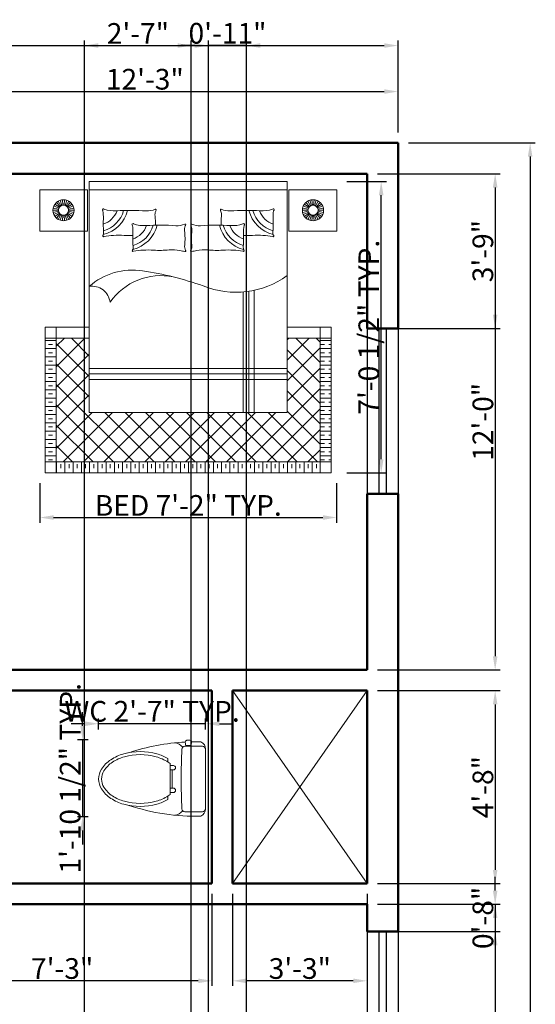
# Model space of a CAD drawing. Units: inches. Extents: x 749 to 1130, y 885 to 1490.
# Tile 5 of 5: x 980 to 1130, y 1204 to 1490. Entities that reach past the tile are written whole.
import ezdxf

# ---------------------------------------------------------------- set-up
doc = ezdxf.new("R2010")
doc.units = ezdxf.units.IN
doc.header["$MEASUREMENT"] = 0
for name, color, linetype, lineweight in [('A-ANNO-DIMS', 2, 'Continuous', 18), ('A-FLOR-FIXT', 9, 'Continuous', 20), ('A-FLOR-OPEN', 1, 'Continuous', 18), ('A-FURN', 9, 'Continuous', 18), ('WALL', 7, 'Continuous', 50), ('WINDOW', 2, 'Continuous', 25)]:
    doc.layers.add(name, color=color, linetype=linetype, lineweight=lineweight)
doc.styles.get("Standard").update_dxf_attribs({"font": 'arial.ttf'})
doc.dimstyles.new('yqi0', dxfattribs={"dimscale": 0, "dimtxt": 6, "dimasz": 4, "dimexe": 1.5, "dimexo": 3, "dimgap": 0.5, "dimtad": 1, "dimdsep": 46, "dimlunit": 4, "dimtxsty": 'Standard', "dimcen": 0, "dimclrd": 256, "dimclre": 256, "dimclrt": 7, "dimadec": 1, "dimazin": 2, "dimtfac": 1, "dimtix": 1, "dimtmove": 2, "dimatfit": 2, "dimfxl": 1, "dimtolj": 1, "dimtzin": 0, "dimarcsym": 0})

# ---------------------------------------------------------------- blocks, each defined once
blk = doc.blocks.new('*D2')
at = {"layer": 'A-ANNO-DIMS', "color": 0, "lineweight": -2, "transparency": 16777216}
for p, q in [((943.07, 1457.46), (943.07, 1470.81)), ((947.07, 1469.31), (1086.07, 1469.31)), ((1090.07, 1457.46), (1090.07, 1470.81))]:
    blk.add_line(p, q, dxfattribs=at)
at = {"layer": 'A-ANNO-DIMS', "color": 0, "transparency": 16777216}
for points in [[(947.07, 1469.98), (947.07, 1468.65), (943.07, 1469.31)], [(1086.07, 1469.98), (1086.07, 1468.65), (1090.07, 1469.31)]]:
    blk.add_solid(points, dxfattribs=at)
at = {"layer": 'Defpoints', "color": 0, "transparency": 16777216}
for p in [(1090.07, 1469.31), (943.07, 1454.46), (1090.07, 1454.46)]:
    blk.add_point(p, dxfattribs=at)
at = {"layer": 'A-ANNO-DIMS', "color": 0, "transparency": 16777216, "insert": (1016.57, 1472.88), "char_height": 6, "attachment_point": 5}
blk.add_mtext('\\A1;12\'-3"', dxfattribs=at)
blk = doc.blocks.new('*D3')
at = {"layer": 'A-ANNO-DIMS', "color": 0, "lineweight": -2, "transparency": 16777216}
for p, q in [((1093.07, 1454.46), (1129.93, 1454.46)), ((1128.43, 1450.46), (1128.43, 918.46)), ((1093.07, 914.46), (1129.93, 914.46))]:
    blk.add_line(p, q, dxfattribs=at)
at = {"layer": 'A-ANNO-DIMS', "color": 0, "transparency": 16777216}
for points in [[(1127.76, 1450.46), (1129.09, 1450.46), (1128.43, 1454.46)], [(1127.76, 918.46), (1129.09, 918.46), (1128.43, 914.46)]]:
    blk.add_solid(points, dxfattribs=at)
at = {"layer": 'Defpoints', "color": 0, "transparency": 16777216}
for p in [(1090.07, 1454.46), (1090.07, 914.46), (1128.43, 914.46)]:
    blk.add_point(p, dxfattribs=at)
at = {"layer": 'A-ANNO-DIMS', "color": 0, "transparency": 16777216, "insert": (1124.88, 1184.46), "char_height": 6, "attachment_point": 5, "rotation": 90}
blk.add_mtext("\\A1;45'", dxfattribs=at)
blk = doc.blocks.new('WD_WIN4')
for p, q in [((-0.5, 0.5), (0.5, 0.5)), ((-0.5, 0.12), (0.5, 0.12)), ((-0.5, -0.12), (0.5, -0.12)), ((-0.5, -0.5), (0.5, -0.5))]:
    blk.add_line(p, q)
blk = doc.blocks.new('yq_matong_01')
for p, q in [((0, 200.5), (0, -200.5)), ((20, 220.5), (138.8, 220.5)), ((252.5, 138), (252.5, 114.5)), ((215.8, 91), (238, 91)), ((238, 104.1), (238, -104.1)), ((215.8, 61), (238, 61)), ((223, 61), (223, -61)), ((215.8, -61), (238, -61)), ((215.8, -91), (238, -91)), ((252.5, -114.5), (252.5, -138)), ((20, -220.5), (138.8, -220.5)), ((97.4, -220.5), (97.4, -225.5)), ((97.4, -225.5), (131.6, -225.5)), ((131.6, -220.5), (131.6, -225.5))]:
    blk.add_line(p, q)
for centre, radius, start, end in [((54.8, 202.4), 54.8, 117.32201, 181.89921), ((20, 200.5), 20, 90, 180), ((63.9, -1165.4), 1416.8, 71.40679, 91.38565), ((138.8, 200.5), 20, 2.30634, 90), ((216.6, 161.2), 83.2, 95.49628, 139.93242), ((-4840.4, 0), 5003.3, 357.69366, 2.30634), ((406.6, -122.9), 283, 105.20877, 123.27785), ((406.6, -122.9), 303, 105.20877, 120.56985), ((439, -242.2), 426.7, 74.79123, 105.20877), ((439, -242.2), 406.7, 74.79123, 105.20877), ((471.4, -122.9), 283, 56.72215, 74.79123), ((471.4, -122.9), 303, 56.72215, 74.79123), ((215.8, 76), 15, 90, 270), ((357.1, -47.5), 192.8, 123.27785, 128.13838), ((520.9, -47.5), 192.8, 32.25649, 56.72215), ((520.9, -47.5), 212.8, 32.25649, 56.72215), ((596.2, 0), 103.8, 360, 32.25649), ((596.2, 0), 123.8, 360, 32.25649), ((215.8, -76), 15, 90, 270), ((520.9, 47.5), 192.8, 303.27785, 327.74351), ((520.9, 47.5), 212.8, 303.27785, 327.74351), ((596.2, 0), 103.8, 327.74351, 360), ((596.2, 0), 123.8, 327.74351, 360), ((357.1, 47.5), 192.8, 231.86162, 236.72215), ((406.6, 122.9), 283, 236.72215, 254.79123), ((471.4, 122.9), 283, 285.20877, 303.27785), ((471.4, 122.9), 303, 285.20877, 303.27785), ((63.9, 1165.4), 1416.8, 272.89667, 288.59321), ((406.6, 122.9), 303, 239.43015, 254.79123), ((439, 242.2), 426.7, 254.79123, 285.20877), ((439, 242.2), 406.7, 254.79123, 285.20877), ((51.3, -204.4), 51.4, 175.68696, 245.09182), ((20, -200.5), 20, 180, 270), ((63.9, 1165.4), 1416.8, 268.61435, 271.20362), ((156.6, -247.4), 63.1, 159.68336, 188.49388), ((114.1, -225.6), 37, 237.52867, 304.27722), ((72.4, -247.4), 63.1, 352.09441, 20.31664), ((138.8, -200.5), 20, 270, 357.69366), ((216.6, -161.2), 83.2, 220.06758, 264.50372)]:
    blk.add_arc(centre, radius, start, end)
blk = doc.blocks.new('BED')
h = blk.add_hatch()
h.set_pattern_fill('TRANS', color=256, scale=12, style=0)
h.set_pattern_definition([(360, (4433.967, -9715.0492), (1e-15, 3), []), (360, (4433.967, -9713.5492), (1e-15, 3), [1.5, -1.5])])
h.paths.add_polyline_path([(48, -103), (52, -103), (52, -58), (48, -58)])
h.paths.add_polyline_path([(-48, -58), (-52, -58), (-52, -103), (-48, -103)])
h = blk.add_hatch()
h.set_pattern_fill('ANSI37', color=256, scale=42, angle=-90, style=0)
h.set_pattern_definition([(315, (7787.1367, 4477.8466), (3.7123106, 3.7123106), []), (45, (7787.1367, 4477.8466), (-3.7123106, 3.7123106), [])])
h.paths.add_polyline_path([(-36, -85), (-36, -58), (-48, -58), (-48, -103), (48, -103), (48, -58), (36, -58), (36, -85)])
h = blk.add_hatch()
h.set_pattern_fill('TRANS', color=256, scale=12, angle=-90, style=0)
h.set_pattern_definition([(270, (4433.967, -9715.0492), (3, -1e-15), []), (270, (4435.467, -9715.0492), (3, -1e-15), [1.5, -1.5])])
h.paths.add_polyline_path([(48, -107), (48, -103), (-48, -103), (-48, -107)])
for p, q in [((-36, -1), (36, -1)), ((-36, -85), (-36, -1)), ((36, -1), (36, -85)), ((-54, -4), (-54, -19)), ((-36.64, -4), (-54, -4)), ((-36.64, -4), (-36.64, -19)), ((-36, -4), (36, -4)), ((36.64, -4), (36.64, -19)), ((36.64, -4), (54, -4)), ((54, -4), (54, -19)), ((-47.19, -11.07), (-49.14, -10.66)), ((-47.07, -10.7), (-48.9, -9.89)), ((-46.88, -10.37), (-48.5, -9.2)), ((-46.62, -10.08), (-47.96, -8.6)), ((-46.31, -9.86), (-47.31, -8.13)), ((-45.96, -9.7), (-46.58, -7.8)), ((-45.58, -9.62), (-45.8, -7.63)), ((-45.2, -9.62), (-45, -7.63)), ((-44.82, -9.7), (-44.21, -7.79)), ((-44.47, -9.85), (-43.48, -8.12)), ((-44.16, -10.08), (-42.83, -8.59)), ((-43.9, -10.36), (-42.29, -9.18)), ((-43.71, -10.7), (-41.89, -9.88)), ((-43.59, -11.06), (-41.64, -10.64)), ((43.59, -11.06), (41.64, -10.64)), ((43.71, -10.7), (41.89, -9.88)), ((43.9, -10.36), (42.29, -9.18)), ((44.16, -10.08), (42.83, -8.59)), ((44.47, -9.85), (43.48, -8.12)), ((44.82, -9.7), (44.21, -7.79)), ((45.2, -9.62), (45, -7.63)), ((45.58, -9.62), (45.8, -7.63)), ((45.96, -9.7), (46.58, -7.8)), ((46.31, -9.86), (47.31, -8.13)), ((46.62, -10.08), (47.96, -8.6)), ((46.88, -10.37), (48.5, -9.2)), ((47.07, -10.7), (48.9, -9.89)), ((47.19, -11.07), (49.14, -10.66)), ((-47.23, -11.45), (-49.23, -11.45)), ((-47.19, -11.83), (-49.14, -12.25)), ((-47.07, -12.2), (-48.89, -13.01)), ((-46.87, -12.53), (-48.49, -13.71)), ((-46.62, -12.81), (-47.95, -14.3)), ((-46.3, -13.04), (-47.3, -14.77)), ((-45.95, -13.2), (-46.57, -15.1)), ((-45.58, -13.27), (-45.78, -15.26)), ((-45.19, -13.27), (-44.98, -15.26)), ((-44.82, -13.19), (-44.2, -15.09)), ((-44.47, -13.04), (-43.46, -14.77)), ((-44.16, -12.81), (-42.82, -14.29)), ((-43.9, -12.52), (-42.28, -13.7)), ((-43.71, -12.19), (-41.88, -13)), ((-43.59, -11.83), (-41.63, -12.24)), ((-43.55, -11.44), (-41.55, -11.44)), ((43.55, -11.44), (41.55, -11.44)), ((43.59, -11.83), (41.63, -12.24)), ((43.71, -12.19), (41.88, -13)), ((43.9, -12.52), (42.28, -13.7)), ((44.16, -12.81), (42.82, -14.29)), ((44.47, -13.04), (43.46, -14.77)), ((44.82, -13.19), (44.2, -15.09)), ((45.19, -13.27), (44.98, -15.26)), ((45.58, -13.27), (45.78, -15.26)), ((45.95, -13.2), (46.57, -15.1)), ((46.3, -13.04), (47.3, -14.77)), ((46.62, -12.81), (47.95, -14.3)), ((46.87, -12.53), (48.49, -13.71)), ((47.07, -12.2), (48.89, -13.01)), ((47.19, -11.83), (49.14, -12.25)), ((47.23, -11.45), (49.23, -11.45)), ((-36.64, -19), (-54, -19)), ((36.64, -19), (54, -19)), ((20, -85), (20, -41.14)), ((22, -85), (22, -40.91)), ((24, -85), (24, -40.55)), ((-52, -54), (-52, -107)), ((-52, -54), (-36, -54)), ((-48, -54), (-48, -107)), ((36, -54), (52, -54)), ((48, -54), (48, -107)), ((52, -54), (52, -107)), ((-52, -58), (-36, -58)), ((36, -58), (52, -58)), ((36, -69), (-36, -69)), ((36, -71), (-36, -71)), ((36, -73), (-36, -73)), ((36, -85), (-36, -85)), ((-52, -103), (52, -103)), ((-52, -107), (52, -107))]:
    blk.add_line(p, q)
for centre, radius in [((-45.39, -11.45), 3.84), ((-45.39, -11.45), 1.84), ((45.39, -11.45), 3.84), ((45.39, -11.45), 1.84)]:
    blk.add_circle(centre, radius)
for centre, radius, start, end in [((-30.92, -11.24), 0.328, 35.8976, 208.6272), ((-42.38, -17.5), 12.73, 27.1629, 28.6272), ((-44.37, -13.89), 13.5, 357.4804, 9.3956), ((-33.8, -8.61), 8.46, 289.8695, 338.9843), ((-33.8, -8.61), 12.06, 283.8498, 346.0842), ((-33.8, -8.61), 10.71, 286.0319, 344.1205), ((-26.84, 0.13), 11.82, 251.1782, 273.3982), ((-20.92, -99.64), 88.13, 86.2964, 93.3982), ((-14.79, -4.98), 6.73, 266.2964, 294.303), ((-8.24, -13.16), 3.86, 159.0146, 186.273), ((-36.64, -16.28), 24.71, 358.5721, 6.273), ((-11.92, -11.33), 0.242, 335.7259, 114.303), ((-5.69, -14.14), 6.59, 155.7259, 159.0146), ((11.92, -11.33), 0.242, 65.697, 204.2741), ((5.69, -14.14), 6.59, 20.9854, 24.2741), ((8.24, -13.16), 3.86, 353.727, 20.9854), ((36.64, -16.28), 24.71, 173.727, 181.4279), ((14.79, -4.98), 6.73, 245.697, 273.7036), ((20.92, -99.64), 88.13, 86.6018, 93.7036), ((33.8, -8.61), 12.06, 193.9158, 256.1502), ((33.8, -8.61), 10.71, 195.8795, 253.9681), ((33.8, -8.61), 8.46, 201.0157, 250.1305), ((26.84, 0.13), 11.82, 266.6018, 288.8218), ((30.92, -11.24), 0.328, 331.3728, 144.1024), ((44.37, -13.89), 13.5, 170.6044, 182.5196), ((42.38, -17.5), 12.73, 151.3728, 152.8371), ((10.15, -16.29), 41.07, 177.4804, 184.5075), ((-20.16, -16.62), 0.328, 35.8976, 208.6272), ((-31.62, -22.87), 12.73, 27.1629, 28.6272), ((-33.61, -19.26), 13.5, 357.4804, 9.3956), ((-23.04, -13.99), 8.46, 289.8695, 338.9843), ((-23.04, -13.99), 12.06, 283.8498, 346.0842), ((-23.04, -13.99), 10.71, 286.0319, 344.1205), ((-16.08, -5.24), 11.82, 251.1782, 273.3982), ((-10.15, -105.01), 88.13, 86.2964, 93.3982), ((-4.03, -10.35), 6.73, 266.2964, 294.303), ((2.52, -18.53), 3.86, 159.0146, 186.273), ((-1.16, -16.7), 0.242, 335.7259, 114.303), ((5.07, -19.51), 6.59, 155.7259, 159.0146), ((1.16, -16.7), 0.242, 65.697, 204.2741), ((-5.07, -19.51), 6.59, 20.9854, 24.2741), ((-2.52, -18.53), 3.86, 353.727, 20.9854), ((4.03, -10.35), 6.73, 245.697, 273.7036), ((10.15, -105.01), 88.13, 86.6018, 93.7036), ((23.04, -13.99), 12.06, 193.9158, 256.1502), ((23.04, -13.99), 10.71, 195.8795, 253.9681), ((23.04, -13.99), 8.46, 201.0157, 250.1305), ((16.08, -5.24), 11.82, 266.6018, 288.8218), ((20.16, -16.62), 0.328, 331.3728, 144.1024), ((33.61, -19.26), 13.5, 170.6044, 182.5196), ((31.62, -22.87), 12.73, 151.3728, 152.8371), ((-10.15, -16.29), 41.07, 355.4925, 2.5196), ((-30.88, -20.82), 0.25, 147.6219, 311.9343), ((-32.72, -19.65), 1.93, 327.6219, 339.2246), ((-32.67, -19.67), 1.88, 339.2246, 4.5075), ((-25.16, -53.53), 33, 93.5164, 99.6766), ((-25.27, -51.86), 31.33, 86.4836, 93.5164), ((-21.12, 15.68), 36.34, 266.4836, 271.5234), ((20.91, -21.66), 41.07, 177.4804, 184.5075), ((-25.88, -21.66), 24.71, 354.3784, 6.273), ((25.88, -21.66), 24.71, 173.727, 185.6216), ((-20.91, -21.66), 41.07, 355.4925, 2.5196), ((21.12, 15.68), 36.34, 268.4766, 273.5164), ((25.27, -51.86), 31.33, 86.4836, 93.5164), ((25.16, -53.53), 33, 80.3234, 86.4836), ((30.88, -20.82), 0.25, 228.0657, 32.3781), ((32.67, -19.67), 1.88, 175.4925, 200.7754), ((32.72, -19.65), 1.93, 200.7754, 212.3781), ((-21.91, -25.04), 1.88, 339.2246, 4.5075), ((2.55, -24.46), 3.86, 174.3784, 204.7617), ((-2.55, -24.46), 3.86, 335.2383, 5.6216), ((21.91, -25.04), 1.88, 175.4925, 200.7754), ((-20.12, -26.19), 0.25, 147.6219, 311.9343), ((-21.96, -25.02), 1.93, 327.6219, 339.2246), ((-14.4, -58.9), 33, 93.5164, 99.6766), ((-14.51, -57.23), 31.33, 86.4836, 93.5164), ((-10.35, 10.3), 36.34, 266.4836, 275.306), ((-5.78, -38.98), 13.15, 77.9645, 95.306), ((2.5, -0.17), 26.53, 257.9645, 261.9243), ((-1.09, -26.25), 0.228, 231.9005, 52.8902), ((1.09, -26.25), 0.228, 127.1098, 308.0995), ((-2.5, -0.17), 26.53, 278.0757, 282.0355), ((5.78, -38.98), 13.15, 84.694, 102.0355), ((10.35, 10.3), 36.34, 264.694, 273.5164), ((14.51, -57.23), 31.33, 86.4836, 93.5164), ((14.4, -58.9), 33, 80.3234, 86.4836), ((20.12, -26.19), 0.25, 228.0657, 32.3781), ((21.96, -25.02), 1.93, 200.7754, 212.3781), ((-20.27, -56.85), 23.66, 81.0857, 131.6581), ((-9.91, -57.83), 22.61, 78.6456, 145.1521), ((-32.56, -143.87), 111.55, 70.0977, 81.7735), ((17.27, -9.21), 32.05, 248.2778, 305.7663), ((-34.97, -45.63), 6.55, 6.3172, 99.0807)]:
    blk.add_arc(centre, radius, start, end)
blk = doc.blocks.new('*D21')
at = {"layer": 'A-ANNO-DIMS', "lineweight": -2, "transparency": 16777216}
for p, q in [((999.16, 1285.87), (995.16, 1285.87)), ((1003.16, 1284.21), (1003.16, 1287.37)), ((1034.22, 1285.87), (1003.16, 1285.87)), ((1034.22, 1284.21), (1034.22, 1287.37)), ((1038.22, 1285.87), (1042.22, 1285.87))]:
    blk.add_line(p, q, dxfattribs=at)
at = {"layer": 'A-ANNO-DIMS', "transparency": 16777216}
for points in [[(999.16, 1286.54), (999.16, 1285.2), (1003.16, 1285.87)], [(1038.22, 1286.54), (1038.22, 1285.2), (1034.22, 1285.87)]]:
    blk.add_solid(points, dxfattribs=at)
at = {"layer": 'Defpoints', "color": 0, "transparency": 16777216}
for p in [(1003.16, 1285.87), (1003.16, 1281.21), (1034.22, 1281.21)]:
    blk.add_point(p, dxfattribs=at)
at = {"layer": 'A-ANNO-DIMS', "color": 7, "transparency": 16777216, "insert": (1018.69, 1289.47), "char_height": 6, "attachment_point": 5}
blk.add_mtext('\\A1;WC 2\'-7" TYP.', dxfattribs=at)
blk = doc.blocks.new('*D22')
at = {"layer": 'A-ANNO-DIMS', "lineweight": -2, "transparency": 16777216}
for p, q in [((998.5, 1285.21), (998.5, 1289.21)), ((1000.16, 1281.21), (997, 1281.21)), ((998.5, 1281.21), (998.5, 1258.84)), ((1000.16, 1258.84), (997, 1258.84)), ((998.5, 1254.84), (998.5, 1250.84))]:
    blk.add_line(p, q, dxfattribs=at)
at = {"layer": 'A-ANNO-DIMS', "transparency": 16777216}
for points in [[(997.83, 1285.21), (999.17, 1285.21), (998.5, 1281.21)], [(997.83, 1254.84), (999.17, 1254.84), (998.5, 1258.84)]]:
    blk.add_solid(points, dxfattribs=at)
at = {"layer": 'Defpoints', "color": 0, "transparency": 16777216}
for p in [(1003.16, 1281.21), (998.5, 1258.84), (1003.16, 1258.84)]:
    blk.add_point(p, dxfattribs=at)
at = {"layer": 'A-ANNO-DIMS', "color": 7, "transparency": 16777216, "insert": (994.9, 1270.02), "char_height": 6, "attachment_point": 5, "rotation": 90}
blk.add_mtext('\\A1;1\'-10 1/2" TYP.', dxfattribs=at)
blk = doc.blocks.new('*D23')
at = {"layer": 'A-ANNO-DIMS', "lineweight": -2, "transparency": 16777216}
for p, q in [((986.09, 1355.63), (986.09, 1344.2)), ((1072.26, 1355.63), (1072.26, 1344.2)), ((990.09, 1345.7), (1068.26, 1345.7))]:
    blk.add_line(p, q, dxfattribs=at)
at = {"layer": 'A-ANNO-DIMS', "transparency": 16777216}
for points in [[(990.09, 1346.37), (990.09, 1345.03), (986.09, 1345.7)], [(1068.26, 1346.37), (1068.26, 1345.03), (1072.26, 1345.7)]]:
    blk.add_solid(points, dxfattribs=at)
at = {"layer": 'Defpoints', "color": 0, "transparency": 16777216}
for p in [(986.09, 1358.63), (1072.26, 1358.63), (1072.26, 1345.7)]:
    blk.add_point(p, dxfattribs=at)
at = {"layer": 'A-ANNO-DIMS', "color": 7, "transparency": 16777216, "insert": (1029.18, 1349.21), "char_height": 6, "attachment_point": 5}
blk.add_mtext('\\A1;BED 7\'-2" TYP.', dxfattribs=at)
blk = doc.blocks.new('*D24')
at = {"layer": 'A-ANNO-DIMS', "lineweight": -2, "transparency": 16777216}
for p, q in [((1075.26, 1443.2), (1086.69, 1443.2)), ((1085.19, 1362.63), (1085.19, 1439.2)), ((1075.26, 1358.63), (1086.69, 1358.63))]:
    blk.add_line(p, q, dxfattribs=at)
at = {"layer": 'A-ANNO-DIMS', "transparency": 16777216}
for points in [[(1084.52, 1439.2), (1085.86, 1439.2), (1085.19, 1443.2)], [(1084.52, 1362.63), (1085.86, 1362.63), (1085.19, 1358.63)]]:
    blk.add_solid(points, dxfattribs=at)
at = {"layer": 'Defpoints', "color": 0, "transparency": 16777216}
for p in [(1072.26, 1443.2), (1085.19, 1443.2), (1072.26, 1358.63)]:
    blk.add_point(p, dxfattribs=at)
at = {"layer": 'A-ANNO-DIMS', "color": 7, "transparency": 16777216, "insert": (1081.59, 1400.92), "char_height": 6, "attachment_point": 5, "rotation": 90}
blk.add_mtext('\\A1;7\'-0 1/2" TYP.', dxfattribs=at)
blk = doc.blocks.new('*D31')
at = {"layer": 'A-ANNO-DIMS', "lineweight": -2, "transparency": 16777216}
for p, q in [((790.07, 1457.46), (790.07, 1484.16)), ((1090.07, 1457.46), (1090.07, 1484.16)), ((794.07, 1482.66), (1086.07, 1482.66))]:
    blk.add_line(p, q, dxfattribs=at)
at = {"layer": 'A-ANNO-DIMS', "transparency": 16777216}
for points in [[(794.07, 1483.33), (794.07, 1481.99), (790.07, 1482.66)], [(1086.07, 1483.33), (1086.07, 1481.99), (1090.07, 1482.66)]]:
    blk.add_solid(points, dxfattribs=at)
at = {"layer": 'Defpoints', "color": 0, "transparency": 16777216}
for p in [(1090.07, 1482.66), (790.07, 1454.46), (1090.07, 1454.46)]:
    blk.add_point(p, dxfattribs=at)
at = {"layer": 'A-ANNO-DIMS', "color": 7, "transparency": 16777216, "insert": (940.07, 1486.22), "char_height": 6, "attachment_point": 5}
blk.add_mtext('\\A1;25\'-0"', dxfattribs=at)
blk = doc.blocks.new('*D36')
at = {"layer": 'A-ANNO-DIMS', "lineweight": -2, "transparency": 16777216}
for p, q in [((1084.07, 1445.46), (1119.77, 1445.46)), ((1118.27, 1441.46), (1118.27, 1305.46)), ((1084.07, 1301.46), (1119.77, 1301.46))]:
    blk.add_line(p, q, dxfattribs=at)
at = {"layer": 'A-ANNO-DIMS', "transparency": 16777216}
for points in [[(1117.6, 1441.46), (1118.94, 1441.46), (1118.27, 1445.46)], [(1117.6, 1305.46), (1118.94, 1305.46), (1118.27, 1301.46)]]:
    blk.add_solid(points, dxfattribs=at)
at = {"layer": 'Defpoints', "color": 0, "transparency": 16777216}
for p in [(1081.07, 1445.46), (1081.07, 1301.46), (1118.27, 1301.46)]:
    blk.add_point(p, dxfattribs=at)
at = {"layer": 'A-ANNO-DIMS', "color": 7, "transparency": 16777216, "insert": (1114.71, 1373.46), "char_height": 6, "attachment_point": 5, "rotation": 90}
blk.add_mtext('\\A1;12\'-0"', dxfattribs=at)
blk = doc.blocks.new('*D37')
at = {"layer": 'A-ANNO-DIMS', "lineweight": -2, "transparency": 16777216}
for p, q in [((1084.07, 1295.46), (1119.77, 1295.46)), ((1118.27, 1291.46), (1118.27, 1243.46)), ((1084.07, 1239.46), (1119.77, 1239.46))]:
    blk.add_line(p, q, dxfattribs=at)
at = {"layer": 'A-ANNO-DIMS', "transparency": 16777216}
for points in [[(1117.6, 1291.46), (1118.94, 1291.46), (1118.27, 1295.46)], [(1117.6, 1243.46), (1118.94, 1243.46), (1118.27, 1239.46)]]:
    blk.add_solid(points, dxfattribs=at)
at = {"layer": 'Defpoints', "color": 0, "transparency": 16777216}
for p in [(1081.07, 1295.46), (1081.07, 1239.46), (1118.27, 1239.46)]:
    blk.add_point(p, dxfattribs=at)
at = {"layer": 'A-ANNO-DIMS', "color": 7, "transparency": 16777216, "insert": (1114.71, 1267.46), "char_height": 6, "attachment_point": 5, "rotation": 90}
blk.add_mtext('\\A1;4\'-8"', dxfattribs=at)
blk = doc.blocks.new('*D38')
at = {"layer": 'A-ANNO-DIMS', "lineweight": -2, "transparency": 16777216}
for p, q in [((1084.07, 1233.46), (1119.77, 1233.46)), ((1118.27, 1229.46), (1118.27, 1093.46)), ((1084.07, 1089.46), (1119.77, 1089.46))]:
    blk.add_line(p, q, dxfattribs=at)
at = {"layer": 'A-ANNO-DIMS', "transparency": 16777216}
for points in [[(1117.6, 1229.46), (1118.94, 1229.46), (1118.27, 1233.46)], [(1117.6, 1093.46), (1118.94, 1093.46), (1118.27, 1089.46)]]:
    blk.add_solid(points, dxfattribs=at)
at = {"layer": 'Defpoints', "color": 0, "transparency": 16777216}
for p in [(1081.07, 1233.46), (1081.07, 1089.46), (1118.27, 1089.46)]:
    blk.add_point(p, dxfattribs=at)
at = {"layer": 'A-ANNO-DIMS', "color": 7, "transparency": 16777216, "insert": (1114.71, 1161.46), "char_height": 6, "attachment_point": 5, "rotation": 90}
blk.add_mtext('\\A1;12\'-0"', dxfattribs=at)
blk = doc.blocks.new('*D48')
at = {"layer": 'A-ANNO-DIMS', "lineweight": -2, "transparency": 16777216}
for p, q in [((999.07, 1087.46), (999.07, 1484.16)), ((1030.07, 1087.46), (1030.07, 1484.16)), ((1003.07, 1482.66), (1026.07, 1482.66))]:
    blk.add_line(p, q, dxfattribs=at)
at = {"layer": 'A-ANNO-DIMS', "transparency": 16777216}
for points in [[(1003.07, 1483.33), (1003.07, 1481.99), (999.07, 1482.66)], [(1026.07, 1483.33), (1026.07, 1481.99), (1030.07, 1482.66)]]:
    blk.add_solid(points, dxfattribs=at)
at = {"layer": 'Defpoints', "color": 0, "transparency": 16777216}
for p in [(1030.07, 1482.66), (999.07, 1084.46), (1030.07, 1084.46)]:
    blk.add_point(p, dxfattribs=at)
at = {"layer": 'A-ANNO-DIMS', "color": 7, "transparency": 16777216, "insert": (1014.57, 1486.17), "char_height": 6, "attachment_point": 5}
blk.add_mtext('\\A1;2\'-7"', dxfattribs=at)
blk = doc.blocks.new('*D50')
at = {"layer": 'A-ANNO-DIMS', "lineweight": -2, "transparency": 16777216}
for p, q in [((1035.07, 1087.46), (1035.07, 1484.16)), ((1046.07, 1087.46), (1046.07, 1484.16)), ((1031.07, 1482.66), (1027.07, 1482.66)), ((1046.07, 1482.66), (1035.07, 1482.66)), ((1050.07, 1482.66), (1054.07, 1482.66))]:
    blk.add_line(p, q, dxfattribs=at)
at = {"layer": 'A-ANNO-DIMS', "transparency": 16777216}
for points in [[(1031.07, 1483.33), (1031.07, 1481.99), (1035.07, 1482.66)], [(1050.07, 1483.33), (1050.07, 1481.99), (1046.07, 1482.66)]]:
    blk.add_solid(points, dxfattribs=at)
at = {"layer": 'Defpoints', "color": 0, "transparency": 16777216}
for p in [(1035.07, 1482.66), (1035.07, 1084.46), (1046.07, 1084.46)]:
    blk.add_point(p, dxfattribs=at)
at = {"layer": 'A-ANNO-DIMS', "color": 7, "transparency": 16777216, "insert": (1040.57, 1486.22), "char_height": 6, "attachment_point": 5}
blk.add_mtext('\\A1;0\'-11"', dxfattribs=at)
blk = doc.blocks.new('*D51')
at = {"layer": 'A-ANNO-DIMS', "lineweight": -2, "transparency": 16777216}
for p, q in [((949.07, 1236.46), (949.07, 1209.76)), ((1036.07, 1236.46), (1036.07, 1209.76)), ((1032.07, 1211.26), (953.07, 1211.26))]:
    blk.add_line(p, q, dxfattribs=at)
at = {"layer": 'A-ANNO-DIMS', "transparency": 16777216}
for points in [[(953.07, 1211.93), (953.07, 1210.59), (949.07, 1211.26)], [(1032.07, 1211.93), (1032.07, 1210.59), (1036.07, 1211.26)]]:
    blk.add_solid(points, dxfattribs=at)
at = {"layer": 'Defpoints', "color": 0, "transparency": 16777216}
for p in [(949.07, 1239.46), (1036.07, 1239.46), (949.07, 1211.26)]:
    blk.add_point(p, dxfattribs=at)
at = {"layer": 'A-ANNO-DIMS', "color": 7, "transparency": 16777216, "insert": (992.57, 1214.83), "char_height": 6, "attachment_point": 5}
blk.add_mtext('\\A1;7\'-3"', dxfattribs=at)
blk = doc.blocks.new('*D52')
at = {"layer": 'A-ANNO-DIMS', "lineweight": -2, "transparency": 16777216}
for p, q in [((1084.07, 1445.46), (1119.77, 1445.46)), ((1118.27, 1441.46), (1118.27, 1404.59)), ((1084.07, 1400.59), (1119.77, 1400.59))]:
    blk.add_line(p, q, dxfattribs=at)
at = {"layer": 'A-ANNO-DIMS', "transparency": 16777216}
for points in [[(1117.6, 1441.46), (1118.94, 1441.46), (1118.27, 1445.46)], [(1117.6, 1404.59), (1118.94, 1404.59), (1118.27, 1400.59)]]:
    blk.add_solid(points, dxfattribs=at)
at = {"layer": 'Defpoints', "color": 0, "transparency": 16777216}
for p in [(1081.07, 1445.46), (1081.07, 1400.59), (1118.27, 1400.59)]:
    blk.add_point(p, dxfattribs=at)
at = {"layer": 'A-ANNO-DIMS', "color": 7, "transparency": 16777216, "insert": (1114.7, 1423.02), "char_height": 6, "attachment_point": 5, "rotation": 90}
blk.add_mtext('\\A1;3\'-9"', dxfattribs=at)
blk = doc.blocks.new('*D53')
at = {"layer": 'A-ANNO-DIMS', "lineweight": -2, "transparency": 16777216}
for p, q in [((1118.27, 1237.46), (1118.27, 1241.46)), ((1084.07, 1233.46), (1119.77, 1233.46)), ((1118.27, 1233.46), (1118.27, 1225.59)), ((1084.07, 1225.59), (1119.77, 1225.59)), ((1118.27, 1221.59), (1118.27, 1217.59))]:
    blk.add_line(p, q, dxfattribs=at)
at = {"layer": 'A-ANNO-DIMS', "transparency": 16777216}
for points in [[(1117.6, 1237.46), (1118.94, 1237.46), (1118.27, 1233.46)], [(1117.6, 1221.59), (1118.94, 1221.59), (1118.27, 1225.59)]]:
    blk.add_solid(points, dxfattribs=at)
at = {"layer": 'Defpoints', "color": 0, "transparency": 16777216}
for p in [(1081.07, 1233.46), (1081.07, 1225.59), (1118.27, 1225.59)]:
    blk.add_point(p, dxfattribs=at)
at = {"layer": 'A-ANNO-DIMS', "color": 7, "transparency": 16777216, "insert": (1114.71, 1229.52), "char_height": 6, "attachment_point": 5, "rotation": 90}
blk.add_mtext('\\A1;0\'-8"', dxfattribs=at)
blk = doc.blocks.new('*D68')
at = {"layer": 'A-ANNO-DIMS', "lineweight": -2, "transparency": 16777216}
for p, q in [((1042.07, 1236.46), (1042.07, 1209.76)), ((1081.07, 1236.46), (1081.07, 1209.76)), ((1077.07, 1211.26), (1046.07, 1211.26))]:
    blk.add_line(p, q, dxfattribs=at)
at = {"layer": 'A-ANNO-DIMS', "transparency": 16777216}
for points in [[(1046.07, 1211.93), (1046.07, 1210.59), (1042.07, 1211.26)], [(1077.07, 1211.93), (1077.07, 1210.59), (1081.07, 1211.26)]]:
    blk.add_solid(points, dxfattribs=at)
at = {"layer": 'Defpoints', "color": 0, "transparency": 16777216}
for p in [(1042.07, 1239.46), (1081.07, 1239.46), (1042.07, 1211.26)]:
    blk.add_point(p, dxfattribs=at)
at = {"layer": 'A-ANNO-DIMS', "color": 7, "transparency": 16777216, "insert": (1061.57, 1214.83), "char_height": 6, "attachment_point": 5}
blk.add_mtext('\\A1;3\'-3"', dxfattribs=at)

msp = doc.modelspace()

# ---------------------------------------------------------------- linework, layer by layer
at = {"layer": 'A-FLOR-OPEN'}
for p, q in [((1042.07, 1295.46), (1081.07, 1239.46)), ((1042.07, 1239.46), (1081.07, 1295.46))]:
    msp.add_line(p, q, dxfattribs=at)
at = {"layer": 'WALL'}
for p, q in [((943.07, 1454.46), (1090.07, 1454.46)), ((1090.07, 1400.586), (1090.07, 1454.46)), ((949.07, 1445.46), (1081.07, 1445.46)), ((1081.07, 1408.46), (1081.07, 1445.46)), ((1081.07, 1400.586), (1081.07, 1408.46)), ((1081.07, 1400.586), (1090.07, 1400.586)), ((1081.07, 1301.46), (1081.07, 1352.586)), ((1081.07, 1352.586), (1090.07, 1352.586)), ((1090.07, 1225.586), (1090.07, 1352.586)), ((949.07, 1301.46), (1073.196, 1301.46)), ((1073.196, 1301.46), (1081.07, 1301.46)), ((949.07, 1295.46), (1036.07, 1295.46)), ((1036.07, 1295.46), (1036.07, 1239.46)), ((1042.07, 1295.46), (1042.07, 1239.46)), ((1042.07, 1295.46), (1073.196, 1295.46)), ((1073.196, 1295.46), (1081.07, 1295.46)), ((1081.07, 1239.46), (1081.07, 1295.46)), ((949.07, 1239.46), (1036.07, 1239.46)), ((1042.07, 1239.46), (1081.07, 1239.46)), ((949.07, 1233.46), (1081.07, 1233.46)), ((1081.07, 1225.586), (1081.07, 1233.46)), ((1081.07, 1225.586), (1090.07, 1225.586))]:
    msp.add_line(p, q, dxfattribs=at)

# ---------------------------------------------------------------- block references
at = {"layer": 'A-FLOR-FIXT', "xscale": 0.0430468521740032, "yscale": 0.0430468521740032, "zscale": 0.0430468521740032, "rotation": 180}
msp.add_blockref('yq_matong_01', (1034.154, 1269.815), dxfattribs=at)
at = {"layer": 'A-FURN', "xscale": 0.797910650636604, "yscale": 0.797910650636604, "zscale": 0.797910650636604}
msp.add_blockref('BED', (1029.177, 1444.002), dxfattribs=at)
at = {"layer": 'WINDOW', "xscale": 48, "zscale": 48}
for p, yscale, rotation in [((1085.57, 1376.586), 9.000000000002274, 270), ((1085.57, 1201.586), 9.000000000001592, 269.9999999999998)]:
    msp.add_blockref('WD_WIN4', p, dxfattribs=dict(at, yscale=yscale, rotation=rotation))

# ---------------------------------------------------------------- dimensions: what is measured, and where the dimension line sits
at = {"layer": 'A-ANNO-DIMS'}
for base, p1, p2, picture, middle in [((1090.07, 1482.66), (790.07, 1454.46), (1090.07, 1454.46), '*D31', (940.07, 1486.224)), ((1030.07, 1482.66), (999.07, 1084.46), (1030.07, 1084.46), '*D48', (1014.57, 1486.173)), ((1035.07, 1482.66), (1046.07, 1084.46), (1035.07, 1084.46), '*D50', (1040.57, 1486.224))]:
    dim = msp.add_linear_dim(base=base, p1=p1, p2=p2, dimstyle='yqi0', override={"dimscale": 1, "dimdec": 1, "dimzin": 1, "dimfrac": 2}, dxfattribs=at)
    dim.commit()
    dim.dimension.update_dxf_attribs({"geometry": picture, "text_midpoint": middle})
for p1, p2, distance, picture, middle in [((943.07, 1454.46), (1090.07, 1454.46), 14.854, '*D2', (1016.57, 1472.88)), ((1090.07, 1454.46), (1090.07, 914.46), 38.358, '*D3', (1124.877, 1184.46))]:
    dim = msp.add_aligned_dim(p1=p1, p2=p2, distance=distance, dimstyle='yqi0', override={"dimscale": 1, "dimclrd": 0, "dimclre": 0, "dimclrt": 0}, dxfattribs=at)
    dim.commit()
    dim.dimension.update_dxf_attribs({"geometry": picture, "text_midpoint": middle})
for base, p1, p2, angle, text, picture, middle in [((1085.19, 1443.204), (1072.264, 1358.626), (1072.264, 1443.204), 90, '<> TYP.', '*D24', (1081.588, 1400.915)), ((1003.16, 1285.869), (1034.223, 1281.209), (1003.16, 1281.209), 180, 'WC <> TYP.', '*D21', (1018.692, 1289.471)), ((998.501, 1258.837), (1003.16, 1281.209), (1003.16, 1258.837), 270, '<> TYP.', '*D22', (994.899, 1270.023))]:
    dim = msp.add_linear_dim(base=base, p1=p1, p2=p2, angle=angle, text=text, dimstyle='yqi0', override={"dimscale": 1, "dimdec": 1, "dimzin": 1, "dimfrac": 2}, dxfattribs=at)
    dim.commit()
    dim.dimension.update_dxf_attribs({"geometry": picture, "text_midpoint": middle})
for base, p1, p2, angle, picture, middle in [((1118.27, 1301.46), (1081.07, 1445.46), (1081.07, 1301.46), 90, '*D36', (1114.706, 1373.46)), ((1118.27, 1400.586), (1081.07, 1445.46), (1081.07, 1400.586), 90, '*D52', (1114.704, 1423.023)), ((1118.27, 1239.46), (1081.07, 1295.46), (1081.07, 1239.46), 90, '*D37', (1114.706, 1267.46)), ((1118.27, 1225.586), (1081.07, 1233.46), (1081.07, 1225.586), 90, '*D53', (1114.706, 1229.523)), ((949.07, 1211.26), (1036.07, 1239.46), (949.07, 1239.46), 180, '*D51', (992.57, 1214.826)), ((1042.07, 1211.26), (1081.07, 1239.46), (1042.07, 1239.46), 180, '*D68', (1061.57, 1214.826)), ((1118.27, 1089.46), (1081.07, 1233.46), (1081.07, 1089.46), 90, '*D38', (1114.706, 1161.46))]:
    dim = msp.add_linear_dim(base=base, p1=p1, p2=p2, angle=angle, dimstyle='yqi0', override={"dimscale": 1, "dimdec": 1, "dimzin": 1, "dimfrac": 2}, dxfattribs=at)
    dim.commit()
    dim.dimension.update_dxf_attribs({"geometry": picture, "text_midpoint": middle})
dim = msp.add_linear_dim(base=(1072.264, 1345.7), p1=(986.089, 1358.626), p2=(1072.264, 1358.626), text='BED <> TYP.', dimstyle='yqi0', override={"dimscale": 1, "dimdec": 1, "dimzin": 1, "dimfrac": 2}, dxfattribs=at)
dim.commit()
dim.dimension.update_dxf_attribs({"geometry": '*D23', "text_midpoint": (1029.177, 1349.214)})

doc.saveas('drawing.dxf')
